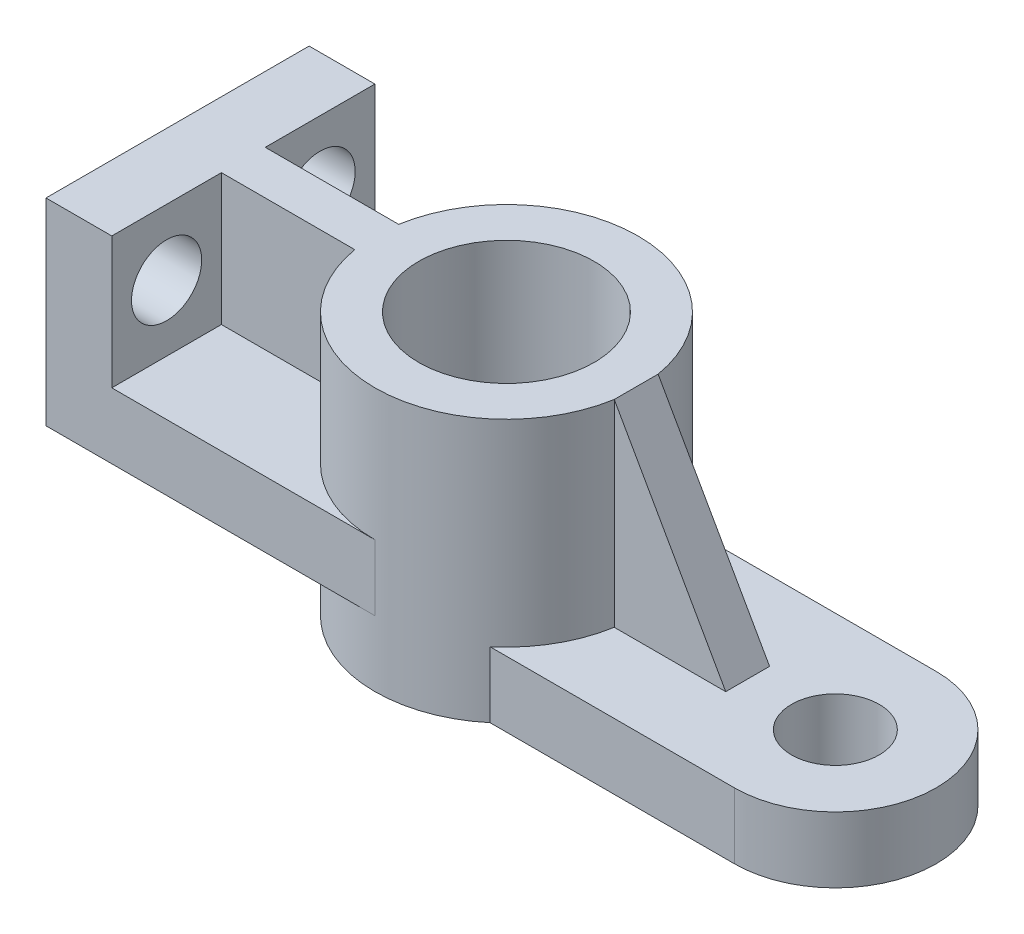
ISO-10303-21;
HEADER;
FILE_DESCRIPTION(('STEP AP214'),'2;1');
FILE_NAME('part.step','',(''),(''),'','','');
FILE_SCHEMA(('AUTOMOTIVE_DESIGN { 1 0 10303 214 1 1 1 1 }'));
ENDSEC;
DATA;
#1=APPLICATION_CONTEXT('core data for automotive mechanical design processes');
#2=APPLICATION_PROTOCOL_DEFINITION('international standard','automotive_design',2000,#1);
#3=PRODUCT_CONTEXT('',#1,'mechanical');
#4=PRODUCT('Part','Part','',(#3));
#5=PRODUCT_RELATED_PRODUCT_CATEGORY('part','',(#4));
#6=PRODUCT_DEFINITION_FORMATION('','',#4);
#7=PRODUCT_DEFINITION_CONTEXT('part definition',#1,'design');
#8=PRODUCT_DEFINITION('design','',#6,#7);
#9=PRODUCT_DEFINITION_SHAPE('','',#8);
#10=(LENGTH_UNIT() NAMED_UNIT(*) SI_UNIT(.MILLI.,.METRE.));
#11=(NAMED_UNIT(*) PLANE_ANGLE_UNIT() SI_UNIT($,.RADIAN.));
#12=(NAMED_UNIT(*) SI_UNIT($,.STERADIAN.) SOLID_ANGLE_UNIT());
#13=UNCERTAINTY_MEASURE_WITH_UNIT(LENGTH_MEASURE(1.E-05),#10,'distance_accuracy_value','');
#14=(GEOMETRIC_REPRESENTATION_CONTEXT(3) GLOBAL_UNCERTAINTY_ASSIGNED_CONTEXT((#13)) GLOBAL_UNIT_ASSIGNED_CONTEXT((#10,
#11,#12)) REPRESENTATION_CONTEXT('',''));
#15=CARTESIAN_POINT('',(0.,0.,0.));
#16=DIRECTION('',(0.,0.,1.));
#17=DIRECTION('',(1.,0.,0.));
#18=AXIS2_PLACEMENT_3D('',#15,#16,#17);
#19=CARTESIAN_POINT('',(0.,30.,30.));
#20=DIRECTION('',(0.,1.,0.));
#21=DIRECTION('',(0.,0.,1.));
#22=AXIS2_PLACEMENT_3D('',#19,#20,#21);
#23=PLANE('',#22);
#24=CARTESIAN_POINT('',(0.,30.,0.));
#25=DIRECTION('',(0.,1.,0.));
#26=DIRECTION('',(0.,0.,1.));
#27=AXIS2_PLACEMENT_3D('',#24,#25,#26);
#28=CIRCLE('',#27,30.);
#29=CARTESIAN_POINT('',(-29.5803989154981,30.,5.));
#30=VERTEX_POINT('',#29);
#31=CARTESIAN_POINT('',(0.,30.,30.));
#32=VERTEX_POINT('',#31);
#33=EDGE_CURVE('E279',#30,#32,#28,.T.);
#34=ORIENTED_EDGE('',*,*,#33,.F.);
#35=DIRECTION('',(1.,0.,0.));
#36=VECTOR('',#35,1.);
#37=CARTESIAN_POINT('',(0.,30.,4.99999999999999));
#38=LINE('',#37,#36);
#39=CARTESIAN_POINT('',(-60.,30.,5.));
#40=VERTEX_POINT('',#39);
#41=EDGE_CURVE('E312',#40,#30,#38,.T.);
#42=ORIENTED_EDGE('',*,*,#41,.F.);
#43=DIRECTION('',(0.,0.,-1.));
#44=VECTOR('',#43,1.);
#45=CARTESIAN_POINT('',(-60.,30.,30.));
#46=LINE('',#45,#44);
#47=CARTESIAN_POINT('',(-60.,30.,30.));
#48=VERTEX_POINT('',#47);
#49=EDGE_CURVE('E271',#48,#40,#46,.T.);
#50=ORIENTED_EDGE('',*,*,#49,.F.);
#51=DIRECTION('',(1.,0.,0.));
#52=VECTOR('',#51,1.);
#53=CARTESIAN_POINT('',(0.,30.,30.));
#54=LINE('',#53,#52);
#55=EDGE_CURVE('E231',#48,#32,#54,.T.);
#56=ORIENTED_EDGE('',*,*,#55,.T.);
#57=EDGE_LOOP('',(#34,#42,#50,#56));
#58=FACE_BOUND('',#57,.T.);
#59=ADVANCED_FACE('F43',(#58),#23,.T.);
#60=CARTESIAN_POINT('',(-60.,0.,30.));
#61=DIRECTION('',(1.,0.,0.));
#62=DIRECTION('',(0.,1.,0.));
#63=AXIS2_PLACEMENT_3D('',#60,#61,#62);
#64=PLANE('',#63);
#65=CARTESIAN_POINT('',(-60.,45.,-17.5));
#66=DIRECTION('',(1.,0.,0.));
#67=DIRECTION('',(0.,1.,0.));
#68=AXIS2_PLACEMENT_3D('',#65,#66,#67);
#69=CIRCLE('',#68,8.);
#70=CARTESIAN_POINT('',(-60.,53.,-17.5));
#71=VERTEX_POINT('',#70);
#72=EDGE_CURVE('E202',#71,#71,#69,.T.);
#73=ORIENTED_EDGE('',*,*,#72,.F.);
#74=EDGE_LOOP('',(#73));
#75=FACE_BOUND('',#74,.T.);
#76=DIRECTION('',(0.,0.,-1.));
#77=VECTOR('',#76,1.);
#78=CARTESIAN_POINT('',(-60.,60.,30.));
#79=LINE('',#78,#77);
#80=CARTESIAN_POINT('',(-60.,60.,-5.));
#81=VERTEX_POINT('',#80);
#82=CARTESIAN_POINT('',(-60.,60.,-30.));
#83=VERTEX_POINT('',#82);
#84=EDGE_CURVE('E268',#81,#83,#79,.T.);
#85=ORIENTED_EDGE('',*,*,#84,.F.);
#86=DIRECTION('',(0.,1.,0.));
#87=VECTOR('',#86,1.);
#88=CARTESIAN_POINT('',(-60.,60.,-5.));
#89=LINE('',#88,#87);
#90=CARTESIAN_POINT('',(-60.,30.,-5.));
#91=VERTEX_POINT('',#90);
#92=EDGE_CURVE('E323',#81,#91,#89,.F.);
#93=ORIENTED_EDGE('',*,*,#92,.T.);
#94=CARTESIAN_POINT('',(-60.,30.,-30.));
#95=VERTEX_POINT('',#94);
#96=EDGE_CURVE('E275',#91,#95,#46,.T.);
#97=ORIENTED_EDGE('',*,*,#96,.T.);
#98=DIRECTION('',(0.,-1.,0.));
#99=VECTOR('',#98,1.);
#100=CARTESIAN_POINT('',(-60.,0.,-30.));
#101=LINE('',#100,#99);
#102=EDGE_CURVE('E253',#83,#95,#101,.T.);
#103=ORIENTED_EDGE('',*,*,#102,.F.);
#104=EDGE_LOOP('',(#85,#93,#97,#103));
#105=FACE_BOUND('',#104,.T.);
#106=ADVANCED_FACE('F353',(#75,#105),#64,.T.);
#107=CARTESIAN_POINT('',(11.5,30.,-5.));
#108=DIRECTION('',(0.,0.,1.));
#109=DIRECTION('',(1.,0.,0.));
#110=AXIS2_PLACEMENT_3D('',#107,#108,#109);
#111=PLANE('',#110);
#112=DIRECTION('',(-0.491834619650922,0.870688639476152,0.));
#113=VECTOR('',#112,1.);
#114=CARTESIAN_POINT('',(55.,15.,-5.));
#115=LINE('',#114,#113);
#116=CARTESIAN_POINT('',(55.,15.,-5.));
#117=VERTEX_POINT('',#116);
#118=CARTESIAN_POINT('',(29.5803989154981,60.,-5.));
#119=VERTEX_POINT('',#118);
#120=EDGE_CURVE('E185',#117,#119,#115,.T.);
#121=ORIENTED_EDGE('',*,*,#120,.F.);
#122=DIRECTION('',(-1.,0.,0.));
#123=VECTOR('',#122,1.);
#124=CARTESIAN_POINT('',(10.,15.,-5.));
#125=LINE('',#124,#123);
#126=CARTESIAN_POINT('',(29.5803989154981,15.,-5.));
#127=VERTEX_POINT('',#126);
#128=EDGE_CURVE('E304',#117,#127,#125,.T.);
#129=ORIENTED_EDGE('',*,*,#128,.T.);
#130=DIRECTION('',(0.,-1.,0.));
#131=VECTOR('',#130,1.);
#132=CARTESIAN_POINT('',(29.5803989154981,60.,-5.));
#133=LINE('',#132,#131);
#134=EDGE_CURVE('E182',#127,#119,#133,.F.);
#135=ORIENTED_EDGE('',*,*,#134,.T.);
#136=EDGE_LOOP('',(#121,#129,#135));
#137=FACE_BOUND('',#136,.T.);
#138=ADVANCED_FACE('F311',(#137),#111,.F.);
#139=CARTESIAN_POINT('',(75.,0.,0.));
#140=DIRECTION('',(0.,1.,0.));
#141=DIRECTION('',(0.,0.,1.));
#142=AXIS2_PLACEMENT_3D('',#139,#140,#141);
#143=CYLINDRICAL_SURFACE('',#142,23.);
#144=DIRECTION('',(0.,-1.,0.));
#145=VECTOR('',#144,1.);
#146=CARTESIAN_POINT('',(75.,0.,-23.));
#147=LINE('',#146,#145);
#148=CARTESIAN_POINT('',(75.,15.,-23.));
#149=VERTEX_POINT('',#148);
#150=CARTESIAN_POINT('',(75.,0.,-23.));
#151=VERTEX_POINT('',#150);
#152=EDGE_CURVE('E296',#149,#151,#147,.T.);
#153=ORIENTED_EDGE('',*,*,#152,.F.);
#154=CARTESIAN_POINT('',(75.,15.,0.));
#155=DIRECTION('',(0.,-1.,0.));
#156=DIRECTION('',(0.,0.,-1.));
#157=AXIS2_PLACEMENT_3D('',#154,#155,#156);
#158=CIRCLE('',#157,23.);
#159=CARTESIAN_POINT('',(75.,15.,23.));
#160=VERTEX_POINT('',#159);
#161=EDGE_CURVE('E303',#160,#149,#158,.F.);
#162=ORIENTED_EDGE('',*,*,#161,.F.);
#163=DIRECTION('',(0.,1.,0.));
#164=VECTOR('',#163,1.);
#165=CARTESIAN_POINT('',(75.,0.,23.));
#166=LINE('',#165,#164);
#167=CARTESIAN_POINT('',(75.,0.,23.));
#168=VERTEX_POINT('',#167);
#169=EDGE_CURVE('E294',#168,#160,#166,.T.);
#170=ORIENTED_EDGE('',*,*,#169,.F.);
#171=CARTESIAN_POINT('',(75.,0.,0.));
#172=DIRECTION('',(0.,1.,0.));
#173=DIRECTION('',(0.,0.,1.));
#174=AXIS2_PLACEMENT_3D('',#171,#172,#173);
#175=CIRCLE('',#174,23.);
#176=EDGE_CURVE('E301',#151,#168,#175,.F.);
#177=ORIENTED_EDGE('',*,*,#176,.F.);
#178=EDGE_LOOP('',(#153,#162,#170,#177));
#179=FACE_BOUND('',#178,.T.);
#180=ADVANCED_FACE('F46',(#179),#143,.T.);
#181=CARTESIAN_POINT('',(0.,60.,0.));
#182=DIRECTION('',(0.,-1.,0.));
#183=DIRECTION('',(0.,0.,-1.));
#184=AXIS2_PLACEMENT_3D('',#181,#182,#183);
#185=CYLINDRICAL_SURFACE('',#184,30.);
#186=CARTESIAN_POINT('',(0.,0.,0.));
#187=DIRECTION('',(0.,1.,0.));
#188=DIRECTION('',(0.,0.,1.));
#189=AXIS2_PLACEMENT_3D('',#186,#187,#188);
#190=CIRCLE('',#189,30.);
#191=CARTESIAN_POINT('',(19.2613602842582,0.,-23.));
#192=VERTEX_POINT('',#191);
#193=CARTESIAN_POINT('',(19.2613602842582,0.,23.));
#194=VERTEX_POINT('',#193);
#195=EDGE_CURVE('E172',#192,#194,#190,.T.);
#196=ORIENTED_EDGE('',*,*,#195,.T.);
#197=DIRECTION('',(0.,-1.,0.));
#198=VECTOR('',#197,1.);
#199=CARTESIAN_POINT('',(19.2613602842582,60.,23.));
#200=LINE('',#199,#198);
#201=CARTESIAN_POINT('',(19.2613602842582,15.,23.));
#202=VERTEX_POINT('',#201);
#203=EDGE_CURVE('E292',#202,#194,#200,.T.);
#204=ORIENTED_EDGE('',*,*,#203,.F.);
#205=CARTESIAN_POINT('',(0.,15.,0.));
#206=DIRECTION('',(0.,-1.,0.));
#207=DIRECTION('',(0.,0.,-1.));
#208=AXIS2_PLACEMENT_3D('',#205,#206,#207);
#209=CIRCLE('',#208,30.);
#210=CARTESIAN_POINT('',(29.5803989154981,15.,5.));
#211=VERTEX_POINT('',#210);
#212=EDGE_CURVE('E191',#211,#202,#209,.T.);
#213=ORIENTED_EDGE('',*,*,#212,.F.);
#214=DIRECTION('',(0.,-1.,0.));
#215=VECTOR('',#214,1.);
#216=CARTESIAN_POINT('',(29.5803989154981,60.,5.));
#217=LINE('',#216,#215);
#218=CARTESIAN_POINT('',(29.5803989154981,60.,5.));
#219=VERTEX_POINT('',#218);
#220=EDGE_CURVE('E186',#211,#219,#217,.F.);
#221=ORIENTED_EDGE('',*,*,#220,.T.);
#222=CARTESIAN_POINT('',(0.,60.,0.));
#223=DIRECTION('',(0.,1.,0.));
#224=DIRECTION('',(0.,0.,1.));
#225=AXIS2_PLACEMENT_3D('',#222,#223,#224);
#226=CIRCLE('',#225,30.);
#227=CARTESIAN_POINT('',(-29.5803989154981,60.,5.));
#228=VERTEX_POINT('',#227);
#229=EDGE_CURVE('E161',#228,#219,#226,.T.);
#230=ORIENTED_EDGE('',*,*,#229,.F.);
#231=DIRECTION('',(0.,-1.,0.));
#232=VECTOR('',#231,1.);
#233=CARTESIAN_POINT('',(-29.5803989154981,60.,5.));
#234=LINE('',#233,#232);
#235=EDGE_CURVE('E316',#30,#228,#234,.F.);
#236=ORIENTED_EDGE('',*,*,#235,.F.);
#237=ORIENTED_EDGE('',*,*,#33,.T.);
#238=DIRECTION('',(0.,-1.,0.));
#239=VECTOR('',#238,1.);
#240=CARTESIAN_POINT('',(0.,0.,30.));
#241=LINE('',#240,#239);
#242=CARTESIAN_POINT('',(0.,15.,30.));
#243=VERTEX_POINT('',#242);
#244=EDGE_CURVE('E233',#32,#243,#241,.T.);
#245=ORIENTED_EDGE('',*,*,#244,.T.);
#246=CARTESIAN_POINT('',(0.,15.,0.));
#247=DIRECTION('',(0.,-1.,0.));
#248=DIRECTION('',(1.,0.,0.));
#249=AXIS2_PLACEMENT_3D('',#246,#247,#248);
#250=CIRCLE('',#249,30.);
#251=CARTESIAN_POINT('',(0.,15.,-30.));
#252=VERTEX_POINT('',#251);
#253=EDGE_CURVE('E277',#243,#252,#250,.T.);
#254=ORIENTED_EDGE('',*,*,#253,.T.);
#255=DIRECTION('',(0.,-1.,0.));
#256=VECTOR('',#255,1.);
#257=CARTESIAN_POINT('',(0.,0.,-30.));
#258=LINE('',#257,#256);
#259=CARTESIAN_POINT('',(0.,30.,-30.));
#260=VERTEX_POINT('',#259);
#261=EDGE_CURVE('E229',#260,#252,#258,.T.);
#262=ORIENTED_EDGE('',*,*,#261,.F.);
#263=CARTESIAN_POINT('',(-29.5803989154981,30.,-5.00000000000001));
#264=VERTEX_POINT('',#263);
#265=EDGE_CURVE('E276',#260,#264,#28,.T.);
#266=ORIENTED_EDGE('',*,*,#265,.T.);
#267=DIRECTION('',(0.,-1.,0.));
#268=VECTOR('',#267,1.);
#269=CARTESIAN_POINT('',(-29.5803989154981,60.,-5.));
#270=LINE('',#269,#268);
#271=CARTESIAN_POINT('',(-29.5803989154981,60.,-5.));
#272=VERTEX_POINT('',#271);
#273=EDGE_CURVE('E322',#264,#272,#270,.F.);
#274=ORIENTED_EDGE('',*,*,#273,.T.);
#275=EDGE_CURVE('E173',#119,#272,#226,.T.);
#276=ORIENTED_EDGE('',*,*,#275,.F.);
#277=ORIENTED_EDGE('',*,*,#134,.F.);
#278=CARTESIAN_POINT('',(19.2613602842582,15.,-23.));
#279=VERTEX_POINT('',#278);
#280=EDGE_CURVE('E226',#279,#127,#209,.T.);
#281=ORIENTED_EDGE('',*,*,#280,.F.);
#282=DIRECTION('',(0.,-1.,0.));
#283=VECTOR('',#282,1.);
#284=CARTESIAN_POINT('',(19.2613602842582,60.,-23.));
#285=LINE('',#284,#283);
#286=EDGE_CURVE('E287',#279,#192,#285,.T.);
#287=ORIENTED_EDGE('',*,*,#286,.T.);
#288=EDGE_LOOP('',(#196,#204,#213,#221,#230,#236,#237,#245,#254,#262,#266,#274,#276,#277,#281,#287));
#289=FACE_BOUND('',#288,.T.);
#290=ADVANCED_FACE('F195',(#289),#185,.T.);
#291=CARTESIAN_POINT('',(0.,60.,0.));
#292=DIRECTION('',(0.,-1.,0.));
#293=DIRECTION('',(0.,0.,-1.));
#294=AXIS2_PLACEMENT_3D('',#291,#292,#293);
#295=CYLINDRICAL_SURFACE('',#294,20.);
#296=CARTESIAN_POINT('',(0.,0.,0.));
#297=DIRECTION('',(0.,1.,0.));
#298=DIRECTION('',(0.,0.,1.));
#299=AXIS2_PLACEMENT_3D('',#296,#297,#298);
#300=CIRCLE('',#299,20.);
#301=CARTESIAN_POINT('',(0.,0.,20.));
#302=VERTEX_POINT('',#301);
#303=EDGE_CURVE('E285',#302,#302,#300,.T.);
#304=ORIENTED_EDGE('',*,*,#303,.F.);
#305=EDGE_LOOP('',(#304));
#306=FACE_BOUND('',#305,.T.);
#307=CARTESIAN_POINT('',(0.,60.,0.));
#308=DIRECTION('',(0.,1.,0.));
#309=DIRECTION('',(0.,0.,1.));
#310=AXIS2_PLACEMENT_3D('',#307,#308,#309);
#311=CIRCLE('',#310,20.);
#312=CARTESIAN_POINT('',(0.,60.,20.));
#313=VERTEX_POINT('',#312);
#314=EDGE_CURVE('E284',#313,#313,#311,.T.);
#315=ORIENTED_EDGE('',*,*,#314,.T.);
#316=EDGE_LOOP('',(#315));
#317=FACE_BOUND('',#316,.T.);
#318=ADVANCED_FACE('F518',(#306,#317),#295,.F.);
#319=CARTESIAN_POINT('',(0.,60.,0.));
#320=DIRECTION('',(0.,1.,0.));
#321=DIRECTION('',(0.,0.,1.));
#322=AXIS2_PLACEMENT_3D('',#319,#320,#321);
#323=PLANE('',#322);
#324=ORIENTED_EDGE('',*,*,#314,.F.);
#325=EDGE_LOOP('',(#324));
#326=FACE_BOUND('',#325,.T.);
#327=ORIENTED_EDGE('',*,*,#229,.T.);
#328=DIRECTION('',(0.,0.,1.));
#329=VECTOR('',#328,1.);
#330=CARTESIAN_POINT('',(29.5803989154981,60.,-30.001));
#331=LINE('',#330,#329);
#332=EDGE_CURVE('E170',#119,#219,#331,.T.);
#333=ORIENTED_EDGE('',*,*,#332,.F.);
#334=ORIENTED_EDGE('',*,*,#275,.T.);
#335=DIRECTION('',(1.,0.,0.));
#336=VECTOR('',#335,1.);
#337=CARTESIAN_POINT('',(-30.,60.,-5.));
#338=LINE('',#337,#336);
#339=EDGE_CURVE('E70',#272,#81,#338,.F.);
#340=ORIENTED_EDGE('',*,*,#339,.T.);
#341=ORIENTED_EDGE('',*,*,#84,.T.);
#342=DIRECTION('',(1.,0.,0.));
#343=VECTOR('',#342,1.);
#344=CARTESIAN_POINT('',(0.,60.,-30.));
#345=LINE('',#344,#343);
#346=CARTESIAN_POINT('',(-75.,60.,-30.));
#347=VERTEX_POINT('',#346);
#348=EDGE_CURVE('E259',#347,#83,#345,.T.);
#349=ORIENTED_EDGE('',*,*,#348,.F.);
#350=DIRECTION('',(0.,0.,-1.));
#351=VECTOR('',#350,1.);
#352=CARTESIAN_POINT('',(-75.,60.,30.));
#353=LINE('',#352,#351);
#354=CARTESIAN_POINT('',(-75.,60.,30.));
#355=VERTEX_POINT('',#354);
#356=EDGE_CURVE('E270',#355,#347,#353,.T.);
#357=ORIENTED_EDGE('',*,*,#356,.F.);
#358=DIRECTION('',(1.,0.,0.));
#359=VECTOR('',#358,1.);
#360=CARTESIAN_POINT('',(0.,60.,30.));
#361=LINE('',#360,#359);
#362=CARTESIAN_POINT('',(-60.,60.,30.));
#363=VERTEX_POINT('',#362);
#364=EDGE_CURVE('E239',#355,#363,#361,.T.);
#365=ORIENTED_EDGE('',*,*,#364,.T.);
#366=CARTESIAN_POINT('',(-60.,60.,5.));
#367=VERTEX_POINT('',#366);
#368=EDGE_CURVE('E269',#363,#367,#79,.T.);
#369=ORIENTED_EDGE('',*,*,#368,.T.);
#370=DIRECTION('',(1.,0.,0.));
#371=VECTOR('',#370,1.);
#372=CARTESIAN_POINT('',(-30.,60.,5.));
#373=LINE('',#372,#371);
#374=EDGE_CURVE('E56',#228,#367,#373,.F.);
#375=ORIENTED_EDGE('',*,*,#374,.F.);
#376=EDGE_LOOP('',(#327,#333,#334,#340,#341,#349,#357,#365,#369,#375));
#377=FACE_BOUND('',#376,.T.);
#378=ADVANCED_FACE('F164',(#326,#377),#323,.T.);
#379=CARTESIAN_POINT('',(0.,0.,0.));
#380=DIRECTION('',(0.,1.,0.));
#381=DIRECTION('',(0.,0.,1.));
#382=AXIS2_PLACEMENT_3D('',#379,#380,#381);
#383=PLANE('',#382);
#384=CARTESIAN_POINT('',(75.,0.,0.));
#385=DIRECTION('',(0.,1.,0.));
#386=DIRECTION('',(0.,0.,1.));
#387=AXIS2_PLACEMENT_3D('',#384,#385,#386);
#388=CIRCLE('',#387,9.99999999999999);
#389=CARTESIAN_POINT('',(75.,0.,9.99999999999999));
#390=VERTEX_POINT('',#389);
#391=EDGE_CURVE('E211',#390,#390,#388,.T.);
#392=ORIENTED_EDGE('',*,*,#391,.T.);
#393=EDGE_LOOP('',(#392));
#394=FACE_BOUND('',#393,.T.);
#395=ORIENTED_EDGE('',*,*,#303,.T.);
#396=EDGE_LOOP('',(#395));
#397=FACE_BOUND('',#396,.T.);
#398=ORIENTED_EDGE('',*,*,#176,.T.);
#399=DIRECTION('',(1.,0.,0.));
#400=VECTOR('',#399,1.);
#401=CARTESIAN_POINT('',(10.,0.,23.));
#402=LINE('',#401,#400);
#403=EDGE_CURVE('E219',#194,#168,#402,.T.);
#404=ORIENTED_EDGE('',*,*,#403,.F.);
#405=ORIENTED_EDGE('',*,*,#195,.F.);
#406=DIRECTION('',(1.,0.,0.));
#407=VECTOR('',#406,1.);
#408=CARTESIAN_POINT('',(10.,0.,-23.));
#409=LINE('',#408,#407);
#410=EDGE_CURVE('E220',#192,#151,#409,.T.);
#411=ORIENTED_EDGE('',*,*,#410,.T.);
#412=EDGE_LOOP('',(#398,#404,#405,#411));
#413=FACE_BOUND('',#412,.T.);
#414=ADVANCED_FACE('F362',(#394,#397,#413),#383,.F.);
#415=DIRECTION('',(1.,0.,0.));
#416=VECTOR('',#415,1.);
#417=CARTESIAN_POINT('',(0.,30.,-5.00000000000001));
#418=LINE('',#417,#416);
#419=EDGE_CURVE('E314',#91,#264,#418,.T.);
#420=ORIENTED_EDGE('',*,*,#419,.T.);
#421=ORIENTED_EDGE('',*,*,#265,.F.);
#422=DIRECTION('',(1.,0.,0.));
#423=VECTOR('',#422,1.);
#424=CARTESIAN_POINT('',(0.,30.,-30.));
#425=LINE('',#424,#423);
#426=EDGE_CURVE('E255',#95,#260,#425,.T.);
#427=ORIENTED_EDGE('',*,*,#426,.F.);
#428=ORIENTED_EDGE('',*,*,#96,.F.);
#429=EDGE_LOOP('',(#420,#421,#427,#428));
#430=FACE_BOUND('',#429,.T.);
#431=ADVANCED_FACE('F358',(#430),#23,.T.);
#432=DIRECTION('',(0.,1.,0.));
#433=VECTOR('',#432,1.);
#434=CARTESIAN_POINT('',(-60.,60.,5.));
#435=LINE('',#434,#433);
#436=EDGE_CURVE('E321',#367,#40,#435,.F.);
#437=ORIENTED_EDGE('',*,*,#436,.F.);
#438=ORIENTED_EDGE('',*,*,#368,.F.);
#439=DIRECTION('',(0.,-1.,0.));
#440=VECTOR('',#439,1.);
#441=CARTESIAN_POINT('',(-60.,0.,30.));
#442=LINE('',#441,#440);
#443=EDGE_CURVE('E240',#363,#48,#442,.T.);
#444=ORIENTED_EDGE('',*,*,#443,.T.);
#445=ORIENTED_EDGE('',*,*,#49,.T.);
#446=EDGE_LOOP('',(#437,#438,#444,#445));
#447=FACE_BOUND('',#446,.T.);
#448=CARTESIAN_POINT('',(-60.,45.,17.5));
#449=DIRECTION('',(1.,0.,0.));
#450=DIRECTION('',(0.,-1.,0.));
#451=AXIS2_PLACEMENT_3D('',#448,#449,#450);
#452=CIRCLE('',#451,8.);
#453=CARTESIAN_POINT('',(-60.,37.,17.5));
#454=VERTEX_POINT('',#453);
#455=EDGE_CURVE('E193',#454,#454,#452,.T.);
#456=ORIENTED_EDGE('',*,*,#455,.F.);
#457=EDGE_LOOP('',(#456));
#458=FACE_BOUND('',#457,.T.);
#459=ADVANCED_FACE('F335',(#447,#458),#64,.T.);
#460=CARTESIAN_POINT('',(-75.,0.,30.));
#461=DIRECTION('',(-1.,0.,0.));
#462=DIRECTION('',(0.,0.,1.));
#463=AXIS2_PLACEMENT_3D('',#460,#461,#462);
#464=PLANE('',#463);
#465=ORIENTED_EDGE('',*,*,#356,.T.);
#466=DIRECTION('',(0.,1.,0.));
#467=VECTOR('',#466,1.);
#468=CARTESIAN_POINT('',(-75.,0.,-30.));
#469=LINE('',#468,#467);
#470=CARTESIAN_POINT('',(-75.,15.,-30.));
#471=VERTEX_POINT('',#470);
#472=EDGE_CURVE('E262',#471,#347,#469,.T.);
#473=ORIENTED_EDGE('',*,*,#472,.F.);
#474=DIRECTION('',(0.,0.,-1.));
#475=VECTOR('',#474,1.);
#476=CARTESIAN_POINT('',(-75.,15.,30.));
#477=LINE('',#476,#475);
#478=CARTESIAN_POINT('',(-75.,15.,30.));
#479=VERTEX_POINT('',#478);
#480=EDGE_CURVE('E248',#479,#471,#477,.T.);
#481=ORIENTED_EDGE('',*,*,#480,.F.);
#482=DIRECTION('',(0.,1.,0.));
#483=VECTOR('',#482,1.);
#484=CARTESIAN_POINT('',(-75.,0.,30.));
#485=LINE('',#484,#483);
#486=EDGE_CURVE('E243',#479,#355,#485,.T.);
#487=ORIENTED_EDGE('',*,*,#486,.T.);
#488=EDGE_LOOP('',(#465,#473,#481,#487));
#489=FACE_BOUND('',#488,.T.);
#490=CARTESIAN_POINT('',(-75.,45.,17.5));
#491=DIRECTION('',(-1.,0.,0.));
#492=DIRECTION('',(0.,0.,1.));
#493=AXIS2_PLACEMENT_3D('',#490,#491,#492);
#494=CIRCLE('',#493,8.);
#495=CARTESIAN_POINT('',(-75.,45.,25.5));
#496=VERTEX_POINT('',#495);
#497=EDGE_CURVE('E199',#496,#496,#494,.F.);
#498=ORIENTED_EDGE('',*,*,#497,.T.);
#499=EDGE_LOOP('',(#498));
#500=FACE_BOUND('',#499,.T.);
#501=CARTESIAN_POINT('',(-75.,45.,-17.5));
#502=DIRECTION('',(-1.,0.,0.));
#503=DIRECTION('',(0.,0.,1.));
#504=AXIS2_PLACEMENT_3D('',#501,#502,#503);
#505=CIRCLE('',#504,8.);
#506=CARTESIAN_POINT('',(-75.,45.,-9.5));
#507=VERTEX_POINT('',#506);
#508=EDGE_CURVE('E210',#507,#507,#505,.F.);
#509=ORIENTED_EDGE('',*,*,#508,.T.);
#510=EDGE_LOOP('',(#509));
#511=FACE_BOUND('',#510,.T.);
#512=ADVANCED_FACE('F341',(#489,#500,#511),#464,.T.);
#513=CARTESIAN_POINT('',(0.,15.,30.));
#514=DIRECTION('',(0.,-1.,0.));
#515=DIRECTION('',(1.,0.,0.));
#516=AXIS2_PLACEMENT_3D('',#513,#514,#515);
#517=PLANE('',#516);
#518=DIRECTION('',(-1.,0.,0.));
#519=VECTOR('',#518,1.);
#520=CARTESIAN_POINT('',(0.,15.,-30.));
#521=LINE('',#520,#519);
#522=EDGE_CURVE('E234',#252,#471,#521,.T.);
#523=ORIENTED_EDGE('',*,*,#522,.F.);
#524=ORIENTED_EDGE('',*,*,#253,.F.);
#525=DIRECTION('',(-1.,0.,0.));
#526=VECTOR('',#525,1.);
#527=CARTESIAN_POINT('',(0.,15.,30.));
#528=LINE('',#527,#526);
#529=EDGE_CURVE('E246',#243,#479,#528,.T.);
#530=ORIENTED_EDGE('',*,*,#529,.T.);
#531=ORIENTED_EDGE('',*,*,#480,.T.);
#532=EDGE_LOOP('',(#523,#524,#530,#531));
#533=FACE_BOUND('',#532,.T.);
#534=ADVANCED_FACE('F346',(#533),#517,.T.);
#535=CARTESIAN_POINT('',(0.,0.,30.));
#536=DIRECTION('',(0.,0.,1.));
#537=DIRECTION('',(1.,0.,0.));
#538=AXIS2_PLACEMENT_3D('',#535,#536,#537);
#539=PLANE('',#538);
#540=ORIENTED_EDGE('',*,*,#244,.F.);
#541=ORIENTED_EDGE('',*,*,#55,.F.);
#542=ORIENTED_EDGE('',*,*,#443,.F.);
#543=ORIENTED_EDGE('',*,*,#364,.F.);
#544=ORIENTED_EDGE('',*,*,#486,.F.);
#545=ORIENTED_EDGE('',*,*,#529,.F.);
#546=EDGE_LOOP('',(#540,#541,#542,#543,#544,#545));
#547=FACE_BOUND('',#546,.T.);
#548=ADVANCED_FACE('F338',(#547),#539,.T.);
#549=CARTESIAN_POINT('',(0.,0.,-30.));
#550=DIRECTION('',(0.,0.,1.));
#551=DIRECTION('',(1.,0.,0.));
#552=AXIS2_PLACEMENT_3D('',#549,#550,#551);
#553=PLANE('',#552);
#554=ORIENTED_EDGE('',*,*,#261,.T.);
#555=ORIENTED_EDGE('',*,*,#522,.T.);
#556=ORIENTED_EDGE('',*,*,#472,.T.);
#557=ORIENTED_EDGE('',*,*,#348,.T.);
#558=ORIENTED_EDGE('',*,*,#102,.T.);
#559=ORIENTED_EDGE('',*,*,#426,.T.);
#560=EDGE_LOOP('',(#554,#555,#556,#557,#558,#559));
#561=FACE_BOUND('',#560,.T.);
#562=ADVANCED_FACE('F407',(#561),#553,.F.);
#563=CARTESIAN_POINT('',(0.,0.,23.));
#564=DIRECTION('',(0.,0.,-1.));
#565=DIRECTION('',(-1.,0.,0.));
#566=AXIS2_PLACEMENT_3D('',#563,#564,#565);
#567=PLANE('',#566);
#568=ORIENTED_EDGE('',*,*,#403,.T.);
#569=ORIENTED_EDGE('',*,*,#169,.T.);
#570=DIRECTION('',(-1.,0.,0.));
#571=VECTOR('',#570,1.);
#572=CARTESIAN_POINT('',(10.,15.,23.));
#573=LINE('',#572,#571);
#574=EDGE_CURVE('E221',#160,#202,#573,.T.);
#575=ORIENTED_EDGE('',*,*,#574,.T.);
#576=ORIENTED_EDGE('',*,*,#203,.T.);
#577=EDGE_LOOP('',(#568,#569,#575,#576));
#578=FACE_BOUND('',#577,.T.);
#579=ADVANCED_FACE('F405',(#578),#567,.F.);
#580=CARTESIAN_POINT('',(0.,0.,-23.));
#581=DIRECTION('',(0.,0.,-1.));
#582=DIRECTION('',(-1.,0.,0.));
#583=AXIS2_PLACEMENT_3D('',#580,#581,#582);
#584=PLANE('',#583);
#585=DIRECTION('',(-1.,0.,0.));
#586=VECTOR('',#585,1.);
#587=CARTESIAN_POINT('',(10.,15.,-23.));
#588=LINE('',#587,#586);
#589=EDGE_CURVE('E225',#149,#279,#588,.T.);
#590=ORIENTED_EDGE('',*,*,#589,.F.);
#591=ORIENTED_EDGE('',*,*,#152,.T.);
#592=ORIENTED_EDGE('',*,*,#410,.F.);
#593=ORIENTED_EDGE('',*,*,#286,.F.);
#594=EDGE_LOOP('',(#590,#591,#592,#593));
#595=FACE_BOUND('',#594,.T.);
#596=ADVANCED_FACE('F403',(#595),#584,.T.);
#597=CARTESIAN_POINT('',(10.,15.,23.));
#598=DIRECTION('',(0.,-1.,0.));
#599=DIRECTION('',(0.,0.,-1.));
#600=AXIS2_PLACEMENT_3D('',#597,#598,#599);
#601=PLANE('',#600);
#602=CARTESIAN_POINT('',(75.,15.,0.));
#603=DIRECTION('',(0.,1.,0.));
#604=DIRECTION('',(0.,0.,1.));
#605=AXIS2_PLACEMENT_3D('',#602,#603,#604);
#606=CIRCLE('',#605,9.99999999999999);
#607=CARTESIAN_POINT('',(75.,15.,9.99999999999999));
#608=VERTEX_POINT('',#607);
#609=EDGE_CURVE('E207',#608,#608,#606,.T.);
#610=ORIENTED_EDGE('',*,*,#609,.F.);
#611=EDGE_LOOP('',(#610));
#612=FACE_BOUND('',#611,.T.);
#613=ORIENTED_EDGE('',*,*,#128,.F.);
#614=DIRECTION('',(0.,0.,-1.));
#615=VECTOR('',#614,1.);
#616=CARTESIAN_POINT('',(55.,15.,23.));
#617=LINE('',#616,#615);
#618=CARTESIAN_POINT('',(55.,15.,5.));
#619=VERTEX_POINT('',#618);
#620=EDGE_CURVE('E55',#117,#619,#617,.F.);
#621=ORIENTED_EDGE('',*,*,#620,.T.);
#622=DIRECTION('',(-1.,0.,0.));
#623=VECTOR('',#622,1.);
#624=CARTESIAN_POINT('',(10.,15.,5.));
#625=LINE('',#624,#623);
#626=EDGE_CURVE('E11',#619,#211,#625,.T.);
#627=ORIENTED_EDGE('',*,*,#626,.T.);
#628=ORIENTED_EDGE('',*,*,#212,.T.);
#629=ORIENTED_EDGE('',*,*,#574,.F.);
#630=ORIENTED_EDGE('',*,*,#161,.T.);
#631=ORIENTED_EDGE('',*,*,#589,.T.);
#632=ORIENTED_EDGE('',*,*,#280,.T.);
#633=EDGE_LOOP('',(#613,#621,#627,#628,#629,#630,#631,#632));
#634=FACE_BOUND('',#633,.T.);
#635=ADVANCED_FACE('F307',(#612,#634),#601,.F.);
#636=CARTESIAN_POINT('',(75.,-31.,0.));
#637=DIRECTION('',(0.,1.,0.));
#638=DIRECTION('',(0.,0.,1.));
#639=AXIS2_PLACEMENT_3D('',#636,#637,#638);
#640=CYLINDRICAL_SURFACE('',#639,9.99999999999999);
#641=ORIENTED_EDGE('',*,*,#391,.F.);
#642=EDGE_LOOP('',(#641));
#643=FACE_BOUND('',#642,.T.);
#644=ORIENTED_EDGE('',*,*,#609,.T.);
#645=EDGE_LOOP('',(#644));
#646=FACE_BOUND('',#645,.T.);
#647=ADVANCED_FACE('F400',(#643,#646),#640,.F.);
#648=CARTESIAN_POINT('',(-75.001,45.,17.5));
#649=DIRECTION('',(1.,0.,0.));
#650=DIRECTION('',(0.,1.,0.));
#651=AXIS2_PLACEMENT_3D('',#648,#649,#650);
#652=CYLINDRICAL_SURFACE('',#651,8.);
#653=ORIENTED_EDGE('',*,*,#497,.F.);
#654=EDGE_LOOP('',(#653));
#655=FACE_BOUND('',#654,.T.);
#656=ORIENTED_EDGE('',*,*,#455,.T.);
#657=EDGE_LOOP('',(#656));
#658=FACE_BOUND('',#657,.T.);
#659=ADVANCED_FACE('F394',(#655,#658),#652,.F.);
#660=CARTESIAN_POINT('',(-75.001,45.,-17.5));
#661=DIRECTION('',(1.,0.,0.));
#662=DIRECTION('',(0.,1.,0.));
#663=AXIS2_PLACEMENT_3D('',#660,#661,#662);
#664=CYLINDRICAL_SURFACE('',#663,8.);
#665=ORIENTED_EDGE('',*,*,#508,.F.);
#666=EDGE_LOOP('',(#665));
#667=FACE_BOUND('',#666,.T.);
#668=ORIENTED_EDGE('',*,*,#72,.T.);
#669=EDGE_LOOP('',(#668));
#670=FACE_BOUND('',#669,.T.);
#671=ADVANCED_FACE('F389',(#667,#670),#664,.F.);
#672=CARTESIAN_POINT('',(11.5,30.,5.));
#673=DIRECTION('',(0.,0.,1.));
#674=DIRECTION('',(1.,0.,0.));
#675=AXIS2_PLACEMENT_3D('',#672,#673,#674);
#676=PLANE('',#675);
#677=DIRECTION('',(0.491834619650922,-0.870688639476152,0.));
#678=VECTOR('',#677,1.);
#679=CARTESIAN_POINT('',(55.,15.,5.));
#680=LINE('',#679,#678);
#681=EDGE_CURVE('E177',#219,#619,#680,.T.);
#682=ORIENTED_EDGE('',*,*,#681,.F.);
#683=ORIENTED_EDGE('',*,*,#220,.F.);
#684=ORIENTED_EDGE('',*,*,#626,.F.);
#685=EDGE_LOOP('',(#682,#683,#684));
#686=FACE_BOUND('',#685,.T.);
#687=ADVANCED_FACE('F189',(#686),#676,.T.);
#688=CARTESIAN_POINT('',(55.,15.,-30.001));
#689=DIRECTION('',(-0.870688639476152,-0.491834619650922,0.));
#690=DIRECTION('',(0.491834619650922,-0.870688639476152,0.));
#691=AXIS2_PLACEMENT_3D('',#688,#689,#690);
#692=PLANE('',#691);
#693=ORIENTED_EDGE('',*,*,#120,.T.);
#694=ORIENTED_EDGE('',*,*,#332,.T.);
#695=ORIENTED_EDGE('',*,*,#681,.T.);
#696=ORIENTED_EDGE('',*,*,#620,.F.);
#697=EDGE_LOOP('',(#693,#694,#695,#696));
#698=FACE_BOUND('',#697,.T.);
#699=ADVANCED_FACE('F178',(#698),#692,.F.);
#700=CARTESIAN_POINT('',(-30.,60.,5.));
#701=DIRECTION('',(0.,0.,1.));
#702=DIRECTION('',(1.,0.,0.));
#703=AXIS2_PLACEMENT_3D('',#700,#701,#702);
#704=PLANE('',#703);
#705=ORIENTED_EDGE('',*,*,#436,.T.);
#706=ORIENTED_EDGE('',*,*,#41,.T.);
#707=ORIENTED_EDGE('',*,*,#235,.T.);
#708=ORIENTED_EDGE('',*,*,#374,.T.);
#709=EDGE_LOOP('',(#705,#706,#707,#708));
#710=FACE_BOUND('',#709,.T.);
#711=ADVANCED_FACE('F328',(#710),#704,.T.);
#712=CARTESIAN_POINT('',(-30.,60.,-5.));
#713=DIRECTION('',(0.,0.,1.));
#714=DIRECTION('',(1.,0.,0.));
#715=AXIS2_PLACEMENT_3D('',#712,#713,#714);
#716=PLANE('',#715);
#717=ORIENTED_EDGE('',*,*,#419,.F.);
#718=ORIENTED_EDGE('',*,*,#92,.F.);
#719=ORIENTED_EDGE('',*,*,#339,.F.);
#720=ORIENTED_EDGE('',*,*,#273,.F.);
#721=EDGE_LOOP('',(#717,#718,#719,#720));
#722=FACE_BOUND('',#721,.T.);
#723=ADVANCED_FACE('F380',(#722),#716,.F.);
#724=CLOSED_SHELL('',(#59,#106,#138,#180,#290,#318,#378,#414,#431,#459,#512,#534,#548,#562,#579,
#596,#635,#647,#659,#671,#687,#699,#711,#723));
#725=MANIFOLD_SOLID_BREP('B2',#724);
#726=ADVANCED_BREP_SHAPE_REPRESENTATION('',(#18,#725),#14);
#727=SHAPE_DEFINITION_REPRESENTATION(#9,#726);
ENDSEC;
END-ISO-10303-21;
